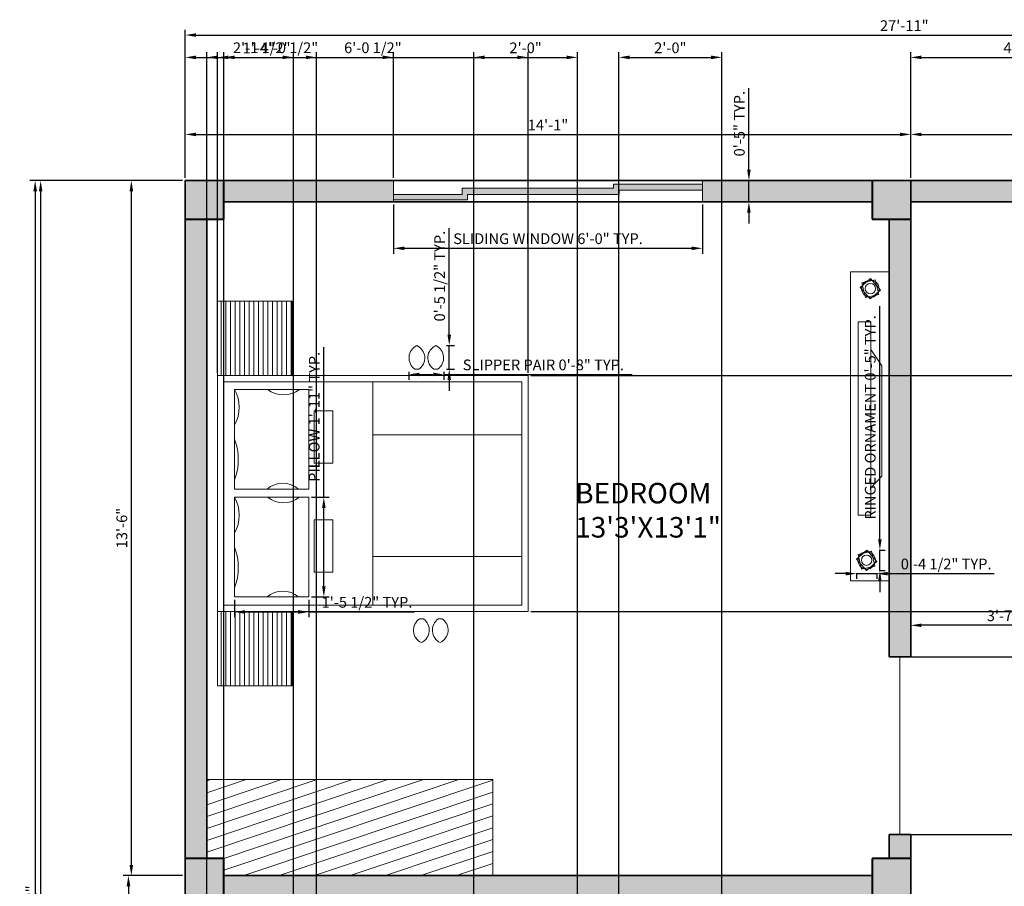
# Model space of a CAD drawing. Units: inches. Extents: x 918 to 1328, y 603 to 1174.
# Tile 3 of 4: x 918 to 1147, y 972 to 1174. Entities that reach past the tile are written whole.
import ezdxf

# ---------------------------------------------------------------- set-up
doc = ezdxf.new("R2010")
doc.units = ezdxf.units.IN
for name, color, linetype, lineweight in [('A-ANNO-DIMS', 1, 'Continuous', 18), ('A-COLS', 7, 'Continuous', 40), ('A-DOOR', 4, 'Continuous', 18), ('A-FLOR-CASE', 8, 'Continuous', 20), ('A-FURN', 8, 'Continuous', 18), ('A-FURN-PATT', 8, 'Continuous', 13), ('A-GLAZ', 4, 'Continuous', 18), ('A-GLAZ-PATT', 5, 'Continuous', 13), ('A-WALL', 7, 'Continuous', 35), ('A-WALL-PATT', 7, 'Continuous', 13)]:
    doc.layers.add(name, color=color, linetype=linetype, lineweight=lineweight)
for name, color, linetype, lineweight, true_color in [('A-AREA-IDEN', 251, 'Continuous', 20, 0x636466), ('A-COLS-PATT', 251, 'Continuous', 13, 0x636466), ('A-EQPM', 252, 'Continuous', 18, 0x939598), ('A-FLOR-CASE-PATT', 251, 'Continuous', 13, 0x636466)]:
    doc.layers.add(name, color=color, linetype=linetype, lineweight=lineweight, true_color=true_color)
doc.styles.get("Standard").update_dxf_attribs({"font": 'arial.ttf'})
doc.dimstyles.new('ISO-25', dxfattribs={"dimtxt": 2.5, "dimasz": 2.5, "dimexe": 1.25, "dimexo": 0.625, "dimtad": 1, "dimdec": 0, "dimlunit": 3, "dimtxsty": 'Standard', "dimcen": 2.5, "dimadec": 0, "dimazin": 0, "dimtfac": 1, "dimtdec": 0, "dimtmove": 0, "dimatfit": 3, "dimfxl": 1, "dimarcsym": 0})

# ---------------------------------------------------------------- blocks, each defined once
blk = doc.blocks.new('*D1')
at = {"layer": 'A-ANNO-DIMS', "color": 0, "lineweight": -2, "transparency": 16777216}
for p, q in [((956.48, 1136.87), (956.48, 1171.39)), ((958.98, 1170.14), (1288.98, 1170.14)), ((1291.48, 1136.87), (1291.48, 1171.39))]:
    blk.add_line(p, q, dxfattribs=at)
at = {"layer": 'A-ANNO-DIMS', "color": 0, "transparency": 16777216}
for points in [[(958.98, 1170.56), (958.98, 1169.73), (956.48, 1170.14)], [(1288.98, 1170.56), (1288.98, 1169.73), (1291.48, 1170.14)]]:
    blk.add_solid(points, dxfattribs=at)
at = {"layer": 'Defpoints', "color": 0, "transparency": 16777216}
for p in [(1291.48, 1170.14), (956.48, 1136.24), (1291.48, 1136.24)]:
    blk.add_point(p, dxfattribs=at)
at = {"layer": 'A-ANNO-DIMS', "color": 0, "transparency": 16777216, "insert": (1123.98, 1172.02), "char_height": 2.5, "attachment_point": 5}
blk.add_mtext('27\'-11"', dxfattribs=at)
blk = doc.blocks.new('*D2')
at = {"layer": 'A-ANNO-DIMS', "color": 0, "lineweight": -2, "transparency": 16777216}
for p, q in [((955.86, 1136.24), (921.53, 1136.24)), ((922.78, 1133.74), (922.78, 800.74)), ((955.86, 798.24), (921.53, 798.24))]:
    blk.add_line(p, q, dxfattribs=at)
at = {"layer": 'A-ANNO-DIMS', "color": 0, "transparency": 16777216}
for points in [[(922.37, 1133.74), (923.2, 1133.74), (922.78, 1136.24)], [(922.37, 800.74), (923.2, 800.74), (922.78, 798.24)]]:
    blk.add_solid(points, dxfattribs=at)
at = {"layer": 'Defpoints', "color": 0, "transparency": 16777216}
for p in [(956.48, 1136.24), (922.78, 798.24), (956.48, 798.24)]:
    blk.add_point(p, dxfattribs=at)
at = {"layer": 'A-ANNO-DIMS', "color": 0, "transparency": 16777216, "insert": (920.88, 967.24), "char_height": 2.5, "attachment_point": 5, "rotation": 90}
blk.add_mtext('28\'-2"', dxfattribs=at)
blk = doc.blocks.new('*D5')
at = {"layer": 'A-ANNO-DIMS', "color": 0, "lineweight": -2, "transparency": 16777216}
for p, q in [((1125.48, 1136.87), (1125.48, 1148.24)), ((1127.98, 1146.99), (1288.98, 1146.99)), ((1291.48, 1136.87), (1291.48, 1148.24))]:
    blk.add_line(p, q, dxfattribs=at)
at = {"layer": 'A-ANNO-DIMS', "color": 0, "transparency": 16777216}
for points in [[(1127.98, 1147.4), (1127.98, 1146.57), (1125.48, 1146.99)], [(1288.98, 1147.4), (1288.98, 1146.57), (1291.48, 1146.99)]]:
    blk.add_solid(points, dxfattribs=at)
at = {"layer": 'Defpoints', "color": 0, "transparency": 16777216}
for p in [(1291.48, 1146.99), (1125.48, 1136.24), (1291.48, 1136.24)]:
    blk.add_point(p, dxfattribs=at)
at = {"layer": 'A-ANNO-DIMS', "color": 0, "transparency": 16777216, "insert": (1208.48, 1148.89), "char_height": 2.5, "attachment_point": 5}
blk.add_mtext('13\'-10"', dxfattribs=at)
blk = doc.blocks.new('*D6')
at = {"layer": 'A-ANNO-DIMS', "color": 0, "lineweight": -2, "transparency": 16777216}
for p, q in [((956.48, 1136.87), (956.48, 1148.24)), ((958.98, 1146.99), (1122.98, 1146.99)), ((1125.48, 1136.87), (1125.48, 1148.24))]:
    blk.add_line(p, q, dxfattribs=at)
at = {"layer": 'A-ANNO-DIMS', "color": 0, "transparency": 16777216}
for points in [[(958.98, 1147.4), (958.98, 1146.57), (956.48, 1146.99)], [(1122.98, 1147.4), (1122.98, 1146.57), (1125.48, 1146.99)]]:
    blk.add_solid(points, dxfattribs=at)
at = {"layer": 'Defpoints', "color": 0, "transparency": 16777216}
for p in [(1125.48, 1146.99), (956.48, 1136.24), (1125.48, 1136.24)]:
    blk.add_point(p, dxfattribs=at)
at = {"layer": 'A-ANNO-DIMS', "color": 0, "transparency": 16777216, "insert": (1040.98, 1148.87), "char_height": 2.5, "attachment_point": 5}
blk.add_mtext('14\'-1"', dxfattribs=at)
blk = doc.blocks.new('*D7')
at = {"layer": 'A-ANNO-DIMS', "color": 0, "lineweight": -2, "transparency": 16777216}
for p, q in [((955.86, 1136.24), (942.66, 1136.24)), ((943.91, 976.74), (943.91, 1133.74)), ((955.86, 974.24), (942.66, 974.24))]:
    blk.add_line(p, q, dxfattribs=at)
at = {"layer": 'A-ANNO-DIMS', "color": 0, "transparency": 16777216}
for points in [[(943.49, 1133.74), (944.33, 1133.74), (943.91, 1136.24)], [(943.49, 976.74), (944.33, 976.74), (943.91, 974.24)]]:
    blk.add_solid(points, dxfattribs=at)
at = {"layer": 'Defpoints', "color": 0, "transparency": 16777216}
for p in [(943.91, 1136.24), (956.48, 1136.24), (956.48, 974.24)]:
    blk.add_point(p, dxfattribs=at)
at = {"layer": 'A-ANNO-DIMS', "color": 0, "transparency": 16777216, "insert": (942.01, 1055.24), "char_height": 2.5, "attachment_point": 5, "rotation": 90}
blk.add_mtext('13\'-6"', dxfattribs=at)
blk = doc.blocks.new('*D8')
at = {"layer": 'A-ANNO-DIMS', "color": 0, "lineweight": -2, "transparency": 16777216}
for p, q in [((955.86, 974.24), (941.99, 974.24)), ((943.24, 971.74), (943.24, 800.74)), ((955.86, 798.24), (941.99, 798.24))]:
    blk.add_line(p, q, dxfattribs=at)
at = {"layer": 'A-ANNO-DIMS', "color": 0, "transparency": 16777216}
for points in [[(942.82, 971.74), (943.66, 971.74), (943.24, 974.24)], [(942.82, 800.74), (943.66, 800.74), (943.24, 798.24)]]:
    blk.add_solid(points, dxfattribs=at)
at = {"layer": 'Defpoints', "color": 0, "transparency": 16777216}
for p in [(956.48, 974.24), (943.24, 798.24), (956.48, 798.24)]:
    blk.add_point(p, dxfattribs=at)
at = {"layer": 'A-ANNO-DIMS', "color": 0, "transparency": 16777216, "insert": (941.34, 886.24), "char_height": 2.5, "attachment_point": 5, "rotation": 90}
blk.add_mtext('14\'-8"', dxfattribs=at)
blk = doc.blocks.new('*D16')
at = {"layer": 'A-ANNO-DIMS', "color": 0, "lineweight": -2, "transparency": 16777216}
for p, q in [((1125.48, 1033.2), (1125.48, 1033.82)), ((1165.98, 1032.57), (1127.98, 1032.57)), ((1168.48, 1033.2), (1168.48, 1033.82))]:
    blk.add_line(p, q, dxfattribs=at)
at = {"layer": 'A-ANNO-DIMS', "color": 0, "transparency": 16777216}
for points in [[(1127.98, 1032.99), (1127.98, 1032.16), (1125.48, 1032.57)], [(1165.98, 1032.99), (1165.98, 1032.16), (1168.48, 1032.57)]]:
    blk.add_solid(points, dxfattribs=at)
at = {"layer": 'Defpoints', "color": 0, "transparency": 16777216}
for p in [(1125.48, 1032.57), (1125.48, 1032.57), (1168.48, 1032.57)]:
    blk.add_point(p, dxfattribs=at)
at = {"layer": 'A-ANNO-DIMS', "color": 0, "transparency": 16777216, "insert": (1146.98, 1034.48), "char_height": 2.5, "attachment_point": 5}
blk.add_mtext('3\'-7"', dxfattribs=at)
blk = doc.blocks.new('WIN-SLIDING-72')
for p, q in [((0, 5), (0, 0)), ((72, 5), (0, 5)), ((72, 0), (72, 5)), ((16, 3.25), (51.22, 3.25)), ((16, 3.25), (16, 1.76)), ((51.22, 4.12), (72, 4.12)), ((51.22, 3.25), (51.22, 4.12)), ((52.58, 2.76), (72, 2.76)), ((52.58, 1.76), (52.58, 2.76)), ((0, 1.76), (16, 1.76)), ((0, 0.47), (17.22, 0.47)), ((0, 0), (72, 0)), ((17.22, 1.76), (51.22, 1.76)), ((17.22, 1.76), (17.22, 0.47)), ((51.22, 1.76), (52.58, 1.76))]:
    blk.add_line(p, q)
blk = doc.blocks.new('PILLOW-BED')
blk.add_lwpolyline([(0, 0), (17.35, 0), (17.35, 23.25), (0, 23.25)], close=True)
for centre, radius, start, end in [((-7.16, 19.07), 8.29, 329.7831, 30.2169), ((11.43, 28.01), 6.06, 231.8235, 308.1765), ((-11.88, 6.88), 12.79, 338.2152, 21.7848), ((11.27, -4.17), 5.55, 48.6314, 131.3686)]:
    blk.add_arc(centre, radius, start, end)
blk = doc.blocks.new('SLIPPERS-PAIR')
for p, q in [((1.4, 0), (2.26, 0)), ((5.79, 0), (6.66, 0))]:
    blk.add_line(p, q)
for centre, start, end in [((3.2, 2.65), 115.3264, 235.7805), ((0.46, 2.65), 304.2195, 64.6736), ((7.59, 2.65), 115.3264, 235.7805), ((4.86, 2.65), 304.2195, 64.6736)]:
    blk.add_arc(centre, 3.2, start, end)
blk = doc.blocks.new('CONSOLE-ORNAMENT-RINGED')
for p, q in [((2.4, 4.76), (0, 2.68)), ((4.73, 2.08), (2.4, 4.76)), ((0, 2.68), (2.33, 0)), ((3.48, 4.49), (0.38, 3.76)), ((0.38, 3.76), (1.19, 0.31)), ((4.29, 1.03), (3.48, 4.49)), ((1.19, 0.31), (4.29, 1.03)), ((2.33, 0), (4.73, 2.08))]:
    blk.add_line(p, q)
for centre, radius in [((2.36, 2.38), 2.02), ((2.35, 2.42), 1.21)]:
    blk.add_circle(centre, radius)
blk = doc.blocks.new('*D30')
at = {"layer": 'A-ANNO-DIMS', "color": 0, "lineweight": -2, "transparency": 16777216}
for p, q in [((1004.98, 1130.62), (1004.98, 1119.19)), ((1076.98, 1130.62), (1076.98, 1119.19)), ((1007.48, 1120.44), (1074.48, 1120.44))]:
    blk.add_line(p, q, dxfattribs=at)
at = {"layer": 'A-ANNO-DIMS', "color": 0, "transparency": 16777216}
for points in [[(1007.48, 1120.86), (1007.48, 1120.03), (1004.98, 1120.44)], [(1074.48, 1120.86), (1074.48, 1120.03), (1076.98, 1120.44)]]:
    blk.add_solid(points, dxfattribs=at)
at = {"layer": 'Defpoints', "color": 0, "transparency": 16777216}
for p in [(1004.98, 1131.24), (1076.98, 1131.24), (1076.98, 1120.44)]:
    blk.add_point(p, dxfattribs=at)
at = {"layer": 'A-ANNO-DIMS', "color": 0, "transparency": 16777216, "insert": (1040.98, 1122.36), "char_height": 2.5, "attachment_point": 5}
blk.add_mtext('SLIDING WINDOW 6\'-0" TYP.', dxfattribs=at)
blk = doc.blocks.new('*D31')
at = {"layer": 'A-ANNO-DIMS', "color": 0, "lineweight": -2, "transparency": 16777216}
for p, q in [((1087.78, 1138.74), (1087.78, 1157.73)), ((1077.61, 1136.24), (1089.03, 1136.24)), ((1087.78, 1131.24), (1087.78, 1136.24)), ((1077.61, 1131.24), (1089.03, 1131.24)), ((1087.78, 1128.74), (1087.78, 1126.24))]:
    blk.add_line(p, q, dxfattribs=at)
at = {"layer": 'A-ANNO-DIMS', "color": 0, "transparency": 16777216}
for points in [[(1087.37, 1138.74), (1088.2, 1138.74), (1087.78, 1136.24)], [(1087.37, 1128.74), (1088.2, 1128.74), (1087.78, 1131.24)]]:
    blk.add_solid(points, dxfattribs=at)
at = {"layer": 'Defpoints', "color": 0, "transparency": 16777216}
for p in [(1076.98, 1136.24), (1087.78, 1136.24), (1076.98, 1131.24)]:
    blk.add_point(p, dxfattribs=at)
at = {"layer": 'A-ANNO-DIMS', "color": 0, "transparency": 16777216, "insert": (1085.88, 1149.49), "char_height": 2.5, "attachment_point": 5, "rotation": 90}
blk.add_mtext('0\'-5" TYP.', dxfattribs=at)
blk = doc.blocks.new('*D36')
at = {"layer": 'A-ANNO-DIMS', "color": 0, "lineweight": -2, "transparency": 16777216}
for p, q in [((988.75, 1062.42), (988.75, 1097.4)), ((985.89, 1062.42), (990, 1062.42)), ((988.75, 1041.68), (988.75, 1059.92)), ((985.89, 1039.18), (990, 1039.18))]:
    blk.add_line(p, q, dxfattribs=at)
at = {"layer": 'A-ANNO-DIMS', "color": 0, "transparency": 16777216}
for points in [[(988.34, 1059.92), (989.17, 1059.92), (988.75, 1062.42)], [(988.34, 1041.68), (989.17, 1041.68), (988.75, 1039.18)]]:
    blk.add_solid(points, dxfattribs=at)
at = {"layer": 'Defpoints', "color": 0, "transparency": 16777216}
for p in [(985.27, 1062.42), (988.75, 1062.42), (985.27, 1039.18)]:
    blk.add_point(p, dxfattribs=at)
at = {"layer": 'A-ANNO-DIMS', "color": 0, "transparency": 16777216, "insert": (986.84, 1081.16), "char_height": 2.5, "attachment_point": 5, "rotation": 90}
blk.add_mtext('PILLOW 1\'-11" TYP.', dxfattribs=at)
blk = doc.blocks.new('*D37')
at = {"layer": 'A-ANNO-DIMS', "color": 0, "lineweight": -2, "transparency": 16777216}
for p, q in [((967.92, 1038.55), (967.92, 1034.44)), ((985.27, 1038.55), (985.27, 1034.44)), ((970.42, 1035.69), (982.77, 1035.69)), ((985.27, 1035.69), (1009.85, 1035.69))]:
    blk.add_line(p, q, dxfattribs=at)
at = {"layer": 'A-ANNO-DIMS', "color": 0, "transparency": 16777216}
for points in [[(970.42, 1036.11), (970.42, 1035.27), (967.92, 1035.69)], [(982.77, 1036.11), (982.77, 1035.27), (985.27, 1035.69)]]:
    blk.add_solid(points, dxfattribs=at)
at = {"layer": 'Defpoints', "color": 0, "transparency": 16777216}
for p in [(967.92, 1039.18), (985.27, 1039.18), (985.27, 1035.69)]:
    blk.add_point(p, dxfattribs=at)
at = {"layer": 'A-ANNO-DIMS', "color": 0, "transparency": 16777216, "insert": (998.81, 1037.61), "char_height": 2.5, "attachment_point": 5}
blk.add_mtext('1\'-5 1/2" TYP.', dxfattribs=at)
blk = doc.blocks.new('*D38')
at = {"layer": 'A-ANNO-DIMS', "color": 0, "lineweight": -2, "transparency": 16777216}
for p, q in [((1008.52, 1091.64), (1008.52, 1089.78)), ((1011.02, 1091.03), (1014.24, 1091.03)), ((1016.74, 1091.64), (1016.74, 1089.78)), ((1016.74, 1091.03), (1060.56, 1091.03))]:
    blk.add_line(p, q, dxfattribs=at)
at = {"layer": 'A-ANNO-DIMS', "color": 0, "transparency": 16777216}
for points in [[(1011.02, 1091.45), (1011.02, 1090.61), (1008.52, 1091.03)], [(1014.24, 1091.45), (1014.24, 1090.61), (1016.74, 1091.03)]]:
    blk.add_solid(points, dxfattribs=at)
at = {"layer": 'Defpoints', "color": 0, "transparency": 16777216}
for p in [(1008.52, 1092.26), (1016.74, 1092.26), (1016.74, 1091.03)]:
    blk.add_point(p, dxfattribs=at)
at = {"layer": 'A-ANNO-DIMS', "color": 0, "transparency": 16777216, "insert": (1039.9, 1092.95), "char_height": 2.5, "attachment_point": 5}
blk.add_mtext('SLIPPER PAIR 0\'-8" TYP.', dxfattribs=at)
blk = doc.blocks.new('*D39')
at = {"layer": 'A-ANNO-DIMS', "color": 0, "lineweight": -2, "transparency": 16777216}
for p, q in [((1017.97, 1100.3), (1017.97, 1125.12)), ((1017.36, 1097.8), (1019.22, 1097.8)), ((1017.97, 1092.26), (1017.97, 1097.8)), ((1017.36, 1092.26), (1019.22, 1092.26)), ((1017.97, 1089.76), (1017.97, 1087.26))]:
    blk.add_line(p, q, dxfattribs=at)
at = {"layer": 'A-ANNO-DIMS', "color": 0, "transparency": 16777216}
for points in [[(1017.55, 1100.3), (1018.39, 1100.3), (1017.97, 1097.8)], [(1017.55, 1089.76), (1018.39, 1089.76), (1017.97, 1092.26)]]:
    blk.add_solid(points, dxfattribs=at)
at = {"layer": 'Defpoints', "color": 0, "transparency": 16777216}
for p in [(1016.74, 1097.8), (1017.97, 1097.8), (1016.74, 1092.26)]:
    blk.add_point(p, dxfattribs=at)
at = {"layer": 'A-ANNO-DIMS', "color": 0, "transparency": 16777216, "insert": (1016.05, 1113.96), "char_height": 2.5, "attachment_point": 5, "rotation": 90}
blk.add_mtext('0\'-5 1/2" TYP.', dxfattribs=at)
blk = doc.blocks.new('*D40')
at = {"layer": 'A-ANNO-DIMS', "color": 0, "lineweight": -2, "transparency": 16777216}
for p, q in [((1118.3, 1052.6), (1118.3, 1106.97)), ((1118.21, 1050.1), (1119.55, 1050.1)), ((1118.3, 1045.33), (1118.3, 1050.1)), ((1118.21, 1045.33), (1119.55, 1045.33)), ((1118.3, 1042.83), (1118.3, 1040.33))]:
    blk.add_line(p, q, dxfattribs=at)
at = {"layer": 'A-ANNO-DIMS', "color": 0, "transparency": 16777216}
for points in [[(1117.88, 1052.6), (1118.71, 1052.6), (1118.3, 1050.1)], [(1117.88, 1042.83), (1118.71, 1042.83), (1118.3, 1045.33)]]:
    blk.add_solid(points, dxfattribs=at)
at = {"layer": 'Defpoints', "color": 0, "transparency": 16777216}
for p in [(1117.58, 1050.1), (1118.3, 1050.1), (1117.58, 1045.33)]:
    blk.add_point(p, dxfattribs=at)
at = {"layer": 'A-ANNO-DIMS', "color": 0, "transparency": 16777216, "insert": (1116.38, 1081.03), "char_height": 2.5, "attachment_point": 5, "rotation": 90}
blk.add_mtext('RINGED ORNAMENT 0\'-5" TYP.', dxfattribs=at)
blk = doc.blocks.new('*D41')
at = {"layer": 'A-ANNO-DIMS', "color": 0, "lineweight": -2, "transparency": 16777216}
for p, q in [((1110.36, 1044.62), (1107.86, 1044.62)), ((1112.86, 1044.71), (1112.86, 1043.37)), ((1112.86, 1044.62), (1117.58, 1044.62)), ((1117.58, 1044.71), (1117.58, 1043.37)), ((1120.08, 1044.62), (1144.9, 1044.62))]:
    blk.add_line(p, q, dxfattribs=at)
at = {"layer": 'A-ANNO-DIMS', "color": 0, "transparency": 16777216}
for points in [[(1110.36, 1045.04), (1110.36, 1044.2), (1112.86, 1044.62)], [(1120.08, 1045.04), (1120.08, 1044.2), (1117.58, 1044.62)]]:
    blk.add_solid(points, dxfattribs=at)
at = {"layer": 'Defpoints', "color": 0, "transparency": 16777216}
for p in [(1112.86, 1045.33), (1117.58, 1045.33), (1117.58, 1044.62)]:
    blk.add_point(p, dxfattribs=at)
at = {"layer": 'A-ANNO-DIMS', "color": 0, "transparency": 16777216, "insert": (1133.74, 1046.54), "char_height": 2.5, "attachment_point": 5}
blk.add_mtext('0\'-4 1/2" TYP.', dxfattribs=at)
blk = doc.blocks.new('*D44')
at = {"layer": 'A-ANNO-DIMS', "color": 0, "lineweight": -2, "transparency": 16777216}
for p, q in [((955.86, 1136.24), (920.25, 1136.24)), ((921.5, 1133.74), (921.5, 731.74)), ((1064.86, 729.24), (920.25, 729.24))]:
    blk.add_line(p, q, dxfattribs=at)
at = {"layer": 'A-ANNO-DIMS', "color": 0, "transparency": 16777216}
for points in [[(921.09, 1133.74), (921.92, 1133.74), (921.5, 1136.24)], [(921.09, 731.74), (921.92, 731.74), (921.5, 729.24)]]:
    blk.add_solid(points, dxfattribs=at)
at = {"layer": 'Defpoints', "color": 0, "transparency": 16777216}
for p in [(956.48, 1136.24), (921.5, 729.24), (1065.48, 729.24)]:
    blk.add_point(p, dxfattribs=at)
at = {"layer": 'A-ANNO-DIMS', "color": 0, "transparency": 16777216, "insert": (919.6, 932.74), "char_height": 2.5, "attachment_point": 5, "rotation": 90}
blk.add_mtext('33\'-11"', dxfattribs=at)
blk = doc.blocks.new('*D45')
at = {"layer": 'A-ANNO-DIMS', "color": 0, "lineweight": -2, "transparency": 16777216}
for p, q in [((956.48, 1136.87), (956.48, 1166.19)), ((1004.98, 1136.87), (1004.98, 1166.19)), ((958.98, 1164.94), (1002.48, 1164.94))]:
    blk.add_line(p, q, dxfattribs=at)
at = {"layer": 'A-ANNO-DIMS', "color": 0, "transparency": 16777216}
for points in [[(958.98, 1165.36), (958.98, 1164.53), (956.48, 1164.94)], [(1002.48, 1165.36), (1002.48, 1164.53), (1004.98, 1164.94)]]:
    blk.add_solid(points, dxfattribs=at)
at = {"layer": 'Defpoints', "color": 0, "transparency": 16777216}
for p in [(1004.98, 1164.94), (956.48, 1136.24), (1004.98, 1136.24)]:
    blk.add_point(p, dxfattribs=at)
at = {"layer": 'A-ANNO-DIMS', "color": 0, "transparency": 16777216, "insert": (980.73, 1166.86), "char_height": 2.5, "attachment_point": 5}
blk.add_mtext('4\'-0 1/2"', dxfattribs=at)
blk = doc.blocks.new('*D46')
at = {"layer": 'A-ANNO-DIMS', "color": 0, "lineweight": -2, "transparency": 16777216}
for p, q in [((1125.48, 1136.87), (1125.48, 1166.19)), ((1176.26, 1136.87), (1176.26, 1166.19)), ((1127.98, 1164.94), (1173.76, 1164.94))]:
    blk.add_line(p, q, dxfattribs=at)
at = {"layer": 'A-ANNO-DIMS', "color": 0, "transparency": 16777216}
for points in [[(1127.98, 1165.36), (1127.98, 1164.53), (1125.48, 1164.94)], [(1173.76, 1165.36), (1173.76, 1164.53), (1176.26, 1164.94)]]:
    blk.add_solid(points, dxfattribs=at)
at = {"layer": 'Defpoints', "color": 0, "transparency": 16777216}
for p in [(1176.26, 1164.94), (1125.48, 1136.24), (1176.26, 1136.24)]:
    blk.add_point(p, dxfattribs=at)
at = {"layer": 'A-ANNO-DIMS', "color": 0, "transparency": 16777216, "insert": (1150.87, 1166.84), "char_height": 2.5, "attachment_point": 5}
blk.add_mtext('4\'-3"', dxfattribs=at)
blk = doc.blocks.new('*D47')
at = {"layer": 'A-ANNO-DIMS', "color": 0, "lineweight": -2, "transparency": 16777216}
for p, q in [((965.48, 803.87), (965.48, 1166.19)), ((981.69, 803.87), (981.69, 1166.19)), ((967.98, 1164.94), (979.19, 1164.94))]:
    blk.add_line(p, q, dxfattribs=at)
at = {"layer": 'A-ANNO-DIMS', "color": 0, "transparency": 16777216}
for points in [[(967.98, 1165.36), (967.98, 1164.53), (965.48, 1164.94)], [(979.19, 1165.36), (979.19, 1164.53), (981.69, 1164.94)]]:
    blk.add_solid(points, dxfattribs=at)
at = {"layer": 'Defpoints', "color": 0, "transparency": 16777216}
for p in [(981.69, 1164.94), (965.48, 803.24), (981.69, 803.24)]:
    blk.add_point(p, dxfattribs=at)
at = {"layer": 'A-ANNO-DIMS', "color": 0, "transparency": 16777216, "insert": (973.59, 1166.82), "char_height": 2.5, "attachment_point": 5}
blk.add_mtext('1\'-4"', dxfattribs=at)
blk = doc.blocks.new('*D48')
at = {"layer": 'A-ANNO-DIMS', "color": 0, "lineweight": -2, "transparency": 16777216}
for p, q in [((1023.69, 803.87), (1023.69, 1166.19)), ((1047.83, 803.87), (1047.83, 1166.19)), ((1026.19, 1164.94), (1045.33, 1164.94))]:
    blk.add_line(p, q, dxfattribs=at)
at = {"layer": 'A-ANNO-DIMS', "color": 0, "transparency": 16777216}
for points in [[(1026.19, 1165.36), (1026.19, 1164.53), (1023.69, 1164.94)], [(1045.33, 1165.36), (1045.33, 1164.53), (1047.83, 1164.94)]]:
    blk.add_solid(points, dxfattribs=at)
at = {"layer": 'Defpoints', "color": 0, "transparency": 16777216}
for p in [(1047.83, 1164.94), (1023.69, 803.24), (1047.83, 803.24)]:
    blk.add_point(p, dxfattribs=at)
at = {"layer": 'A-ANNO-DIMS', "color": 0, "transparency": 16777216, "insert": (1035.76, 1166.84), "char_height": 2.5, "attachment_point": 5}
blk.add_mtext('2\'-0"', dxfattribs=at)
blk = doc.blocks.new('*D50')
at = {"layer": 'A-ANNO-DIMS', "color": 0, "lineweight": -2, "transparency": 16777216}
for p, q in [((1121.11, 1025.24), (1321.43, 1025.24)), ((1320.18, 1022.74), (1320.18, 986.29)), ((1121.11, 983.79), (1321.43, 983.79))]:
    blk.add_line(p, q, dxfattribs=at)
at = {"layer": 'A-ANNO-DIMS', "color": 0, "transparency": 16777216}
for points in [[(1319.77, 1022.74), (1320.6, 1022.74), (1320.18, 1025.24)], [(1319.77, 986.29), (1320.6, 986.29), (1320.18, 983.79)]]:
    blk.add_solid(points, dxfattribs=at)
at = {"layer": 'Defpoints', "color": 0, "transparency": 16777216}
for p in [(1120.48, 1025.24), (1120.48, 983.79), (1320.18, 983.79)]:
    blk.add_point(p, dxfattribs=at)
at = {"layer": 'A-ANNO-DIMS', "color": 0, "transparency": 16777216, "insert": (1318.26, 1004.52), "char_height": 2.5, "attachment_point": 5, "rotation": 90}
blk.add_mtext('3\'-5 1/2"', dxfattribs=at)
blk = doc.blocks.new('*D52')
at = {"layer": 'A-ANNO-DIMS', "color": 0, "lineweight": -2, "transparency": 16777216}
for p, q in [((964.01, 1091.42), (964.01, 1166.19)), ((1036.36, 1091.42), (1036.36, 1166.19)), ((966.51, 1164.94), (1033.86, 1164.94))]:
    blk.add_line(p, q, dxfattribs=at)
at = {"layer": 'A-ANNO-DIMS', "color": 0, "transparency": 16777216}
for points in [[(966.51, 1165.36), (966.51, 1164.53), (964.01, 1164.94)], [(1033.86, 1165.36), (1033.86, 1164.53), (1036.36, 1164.94)]]:
    blk.add_solid(points, dxfattribs=at)
at = {"layer": 'Defpoints', "color": 0, "transparency": 16777216}
for p in [(1036.36, 1164.94), (964.01, 1090.79), (1036.36, 1090.79)]:
    blk.add_point(p, dxfattribs=at)
at = {"layer": 'A-ANNO-DIMS', "color": 0, "transparency": 16777216, "insert": (1000.18, 1166.86), "char_height": 2.5, "attachment_point": 5}
blk.add_mtext('6\'-0 1/2"', dxfattribs=at)
blk = doc.blocks.new('*D53')
at = {"layer": 'A-ANNO-DIMS', "color": 0, "lineweight": -2, "transparency": 16777216}
for p, q in [((1036.99, 1090.79), (1321.43, 1090.79)), ((1320.18, 1038.3), (1320.18, 1088.29)), ((1036.99, 1035.8), (1321.43, 1035.8))]:
    blk.add_line(p, q, dxfattribs=at)
at = {"layer": 'A-ANNO-DIMS', "color": 0, "transparency": 16777216}
for points in [[(1319.77, 1088.29), (1320.6, 1088.29), (1320.18, 1090.79)], [(1319.77, 1038.3), (1320.6, 1038.3), (1320.18, 1035.8)]]:
    blk.add_solid(points, dxfattribs=at)
at = {"layer": 'Defpoints', "color": 0, "transparency": 16777216}
for p in [(1036.36, 1090.79), (1320.18, 1090.79), (1036.36, 1035.8)]:
    blk.add_point(p, dxfattribs=at)
at = {"layer": 'A-ANNO-DIMS', "color": 0, "transparency": 16777216, "insert": (1318.31, 1063.3), "char_height": 2.5, "attachment_point": 5, "rotation": 90}
blk.add_mtext('4\'-7"', dxfattribs=at)
blk = doc.blocks.new('*D54')
at = {"layer": 'A-ANNO-DIMS', "color": 0, "lineweight": -2, "transparency": 16777216}
for p, q in [((961.48, 868.87), (961.48, 1166.19)), ((987.08, 868.87), (987.08, 1166.19)), ((963.98, 1164.94), (984.58, 1164.94))]:
    blk.add_line(p, q, dxfattribs=at)
at = {"layer": 'A-ANNO-DIMS', "color": 0, "transparency": 16777216}
for points in [[(963.98, 1165.36), (963.98, 1164.53), (961.48, 1164.94)], [(984.58, 1165.36), (984.58, 1164.53), (987.08, 1164.94)]]:
    blk.add_solid(points, dxfattribs=at)
at = {"layer": 'Defpoints', "color": 0, "transparency": 16777216}
for p in [(987.08, 1164.94), (961.48, 868.24), (987.08, 868.24)]:
    blk.add_point(p, dxfattribs=at)
at = {"layer": 'A-ANNO-DIMS', "color": 0, "transparency": 16777216, "insert": (974.28, 1166.86), "char_height": 2.5, "attachment_point": 5}
blk.add_mtext('2\'-1 1/2"', dxfattribs=at)
blk = doc.blocks.new('*D55')
at = {"layer": 'A-ANNO-DIMS', "color": 0, "lineweight": -2, "transparency": 16777216}
for p, q in [((1057.48, 856.87), (1057.48, 1166.19)), ((1081.48, 856.87), (1081.48, 1166.19)), ((1059.98, 1164.94), (1078.98, 1164.94))]:
    blk.add_line(p, q, dxfattribs=at)
at = {"layer": 'A-ANNO-DIMS', "color": 0, "transparency": 16777216}
for points in [[(1059.98, 1165.36), (1059.98, 1164.53), (1057.48, 1164.94)], [(1078.98, 1165.36), (1078.98, 1164.53), (1081.48, 1164.94)]]:
    blk.add_solid(points, dxfattribs=at)
at = {"layer": 'Defpoints', "color": 0, "transparency": 16777216}
for p in [(1081.48, 1164.94), (1057.48, 856.24), (1081.48, 856.24)]:
    blk.add_point(p, dxfattribs=at)
at = {"layer": 'A-ANNO-DIMS', "color": 0, "transparency": 16777216, "insert": (1069.48, 1166.84), "char_height": 2.5, "attachment_point": 5}
blk.add_mtext('2\'-0"', dxfattribs=at)

msp = doc.modelspace()

# ---------------------------------------------------------------- hatches: boundary and pattern name
at = {"layer": 'A-COLS-PATT'}
h = msp.add_hatch(color=256, dxfattribs=at)
h.dxf.hatch_style = 1
h.paths.add_polyline_path([(965.48, 1136.24), (956.48, 1136.24), (956.48, 1127.24), (965.48, 1127.24)])
h.paths.add_polyline_path([(1125.48, 1136.24), (1116.48, 1136.24), (1116.48, 1127.24), (1125.48, 1127.24)])
h.paths.add_polyline_path([(1291.48, 1136.24), (1282.48, 1136.24), (1282.48, 1127.24), (1291.48, 1127.24)])
h.paths.add_polyline_path([(1125.48, 978.24), (1116.48, 978.24), (1116.48, 969.24), (1125.48, 969.24)])
h.paths.add_polyline_path([(965.48, 978.24), (956.48, 978.24), (956.48, 969.24), (965.48, 969.24)])
h.paths.add_polyline_path([(965.48, 807.24), (956.48, 807.24), (956.48, 798.24), (965.48, 798.24)])
h.paths.add_polyline_path([(1125.48, 807.24), (1116.48, 807.24), (1116.48, 798.24), (1125.48, 798.24)])
h.paths.add_polyline_path([(1291.48, 807.24), (1282.48, 807.24), (1282.48, 798.24), (1291.48, 798.24)])
h.paths.add_polyline_path([(1291.48, 1030.24), (1282.48, 1030.24), (1282.48, 1021.24), (1291.48, 1021.24)])
h.paths.add_polyline_path([(1291.48, 978.24), (1282.48, 978.24), (1282.48, 969.24), (1291.48, 969.24)])
at = {"layer": 'A-FLOR-CASE-PATT'}
h = msp.add_hatch(dxfattribs=at)
h.set_pattern_fill('ANSI31', color=256, scale=0.827794, angle=-26.45, style=0)
h.paths.add_polyline_path([(961.48, 978.24), (965.48, 978.24), (965.48, 974.24), (1028.14, 974.24), (1028.14, 996.61), (961.48, 996.61)])
at = {"layer": 'A-FURN-PATT'}
h = msp.add_hatch(dxfattribs=at)
h.set_pattern_fill('ANSI31', color=256, scale=0.3418386, angle=45, style=0)
h.paths.add_polyline_path([(964.01, 1090.79), (981.37, 1090.79), (981.37, 1108.16), (964.01, 1108.16)])
h = msp.add_hatch(dxfattribs=at)
h.set_pattern_fill('ANSI31', color=256, scale=0.3418386, angle=45, style=0)
h.paths.add_polyline_path([(964.01, 1018.44), (981.37, 1018.44), (981.37, 1035.8), (964.01, 1035.8)])
at = {"layer": 'A-GLAZ-PATT'}
h = msp.add_hatch(color=256, dxfattribs=at)
h.dxf.hatch_style = 1
h.paths.add_polyline_path([(1057.57, 1134.01), (1076.98, 1134.01), (1076.98, 1135.36), (1056.2, 1135.36), (1056.2, 1134.49), (1020.98, 1134.49), (1020.98, 1133), (1004.98, 1133), (1004.98, 1131.71), (1022.21, 1131.71), (1022.21, 1133), (1056.21, 1133), (1057.57, 1133)])
h.paths.add_polyline_path([(1228.84, 1134.01), (1248.26, 1134.01), (1248.26, 1135.36), (1227.48, 1135.36), (1227.48, 1134.49), (1192.26, 1134.49), (1192.26, 1133), (1176.26, 1133), (1176.26, 1131.71), (1193.48, 1131.71), (1193.48, 1133), (1227.48, 1133), (1228.84, 1133)])
h.paths.add_polyline_path([(1244.5, 828.01), (1263.92, 828.01), (1263.92, 829.36), (1243.14, 829.36), (1243.14, 828.49), (1207.92, 828.49), (1207.92, 827), (1191.92, 827), (1191.92, 825.71), (1209.14, 825.71), (1209.14, 827), (1243.14, 827), (1244.5, 827)])
at = {"layer": 'A-WALL-PATT'}
h = msp.add_hatch(color=256, dxfattribs=at)
h.dxf.hatch_style = 1
h.paths.add_polyline_path([(961.48, 969.24), (956.48, 969.24), (956.48, 807.24), (961.48, 807.24), (961.48, 904.24), (1125.48, 904.24), (1125.48, 909.24), (1086.48, 909.24), (1086.48, 913.24), (1081.48, 913.24), (1081.48, 909.24), (961.48, 909.24)])
h.paths.add_polyline_path([(1116.48, 974.24), (965.48, 974.24), (965.48, 969.24), (1081.48, 969.24), (1081.48, 943.24), (1086.48, 943.24), (1086.48, 969.24), (1116.48, 969.24)])
h.paths.add_polyline_path([(1004.98, 1136.24), (965.48, 1136.24), (965.48, 1131.24), (1004.98, 1131.24)])
h.paths.add_polyline_path([(1116.48, 1136.24), (1076.98, 1136.24), (1076.98, 1131.24), (1116.48, 1131.24)])
h.paths.add_polyline_path([(1176.26, 1136.24), (1125.48, 1136.24), (1125.48, 1131.24), (1176.26, 1131.24)])
h.paths.add_polyline_path([(1282.48, 1136.24), (1248.26, 1136.24), (1248.26, 1131.24), (1282.48, 1131.24)])
h.paths.add_polyline_path([(1125.48, 1127.24), (1120.48, 1127.24), (1120.48, 1025.24), (1125.48, 1025.24)])
h.paths.add_polyline_path([(1291.48, 1035.24), (1168.48, 1035.24), (1168.48, 1030.24), (1291.48, 1030.24)])
h.paths.add_polyline_path([(1125.48, 825.24), (1129.48, 825.24), (1129.48, 830.24), (1125.48, 830.24), (1125.48, 856.24), (1120.48, 856.24), (1120.48, 807.24), (1125.48, 807.24)])
h.paths.add_polyline_path([(1191.92, 830.24), (1177.48, 830.24), (1177.48, 825.24), (1191.92, 825.24)])
h.paths.add_polyline_path([(1291.48, 969.24), (1286.48, 969.24), (1286.48, 830.24), (1263.92, 830.24), (1263.92, 825.24), (1286.48, 825.24), (1286.48, 807.24), (1291.48, 807.24)])
h.paths.add_polyline_path([(1291.48, 1021.24), (1286.48, 1021.24), (1286.48, 978.24), (1291.48, 978.24)])
h.paths.add_polyline_path([(1291.48, 1127.24), (1286.48, 1127.24), (1286.48, 1035.24), (1291.48, 1035.24)])
h = msp.add_hatch(color=256, dxfattribs=at)
h.dxf.hatch_style = 1
h.paths.add_polyline_path([(961.48, 1127.24), (956.48, 1127.24), (956.48, 978.24), (961.48, 978.24), (961.48, 996.61)])
h = msp.add_hatch(color=256, dxfattribs=at)
h.dxf.hatch_style = 1
h.paths.add_polyline_path([(1125.48, 983.79), (1120.48, 983.79), (1120.48, 978.24), (1125.48, 978.24)])

# ---------------------------------------------------------------- linework, layer by layer
at = {"layer": 'A-COLS'}
for p, q in [((965.48, 1127.24), (965.48, 1136.24)), ((1116.48, 1136.24), (1116.48, 1127.24)), ((956.48, 1127.24), (965.48, 1127.24)), ((1116.48, 1127.24), (1125.48, 1127.24)), ((965.48, 978.24), (956.48, 978.24)), ((965.48, 969.24), (965.48, 978.24)), ((1125.48, 978.24), (1116.48, 978.24)), ((1116.48, 978.24), (1116.48, 969.24))]:
    msp.add_line(p, q, dxfattribs=at)
at = {"layer": 'A-DOOR'}
msp.add_line((1122.98, 983.79), (1122.98, 1025.24), dxfattribs=at)
at = {"layer": 'A-EQPM'}
for p, q in [((1116.16, 1103.3), (1113.21, 1103.3)), ((1113.21, 1103.3), (1113.21, 1058.22)), ((1116.16, 1058.22), (1116.16, 1103.3)), ((1116.16, 1096.89), (1118.76, 1093.02)), ((1118.76, 1093.02), (1118.76, 1067.31)), ((1118.76, 1067.31), (1116.16, 1064.61)), ((1113.21, 1058.22), (1116.16, 1058.22))]:
    msp.add_line(p, q, dxfattribs=at)
at = {"layer": 'A-FLOR-CASE'}
for p, q in [((1120.48, 1114.95), (1111.48, 1114.95)), ((1111.48, 1114.95), (1111.48, 1042.95)), ((1120.48, 1042.95), (1120.48, 1114.95)), ((1111.48, 1042.95), (1120.48, 1042.95)), ((961.48, 996.61), (961.48, 978.24)), ((1028.14, 996.61), (961.48, 996.61)), ((1028.14, 974.24), (1028.14, 996.61)), ((965.48, 974.24), (1028.14, 974.24))]:
    msp.add_line(p, q, dxfattribs=at)
at = {"layer": 'A-FURN'}
for p, q in [((1000.18, 1089.35), (1000.18, 1037.25)), ((976.99, 1035.8), (964.01, 1035.8)), ((964.01, 1035.8), (964.01, 1018.44)), ((981.37, 1035.8), (981.37, 1018.44)), ((964.01, 1018.44), (981.37, 1018.44))]:
    msp.add_line(p, q, dxfattribs=at)
for points in [[(964.01, 1090.79), (981.37, 1090.79), (981.37, 1108.16), (964.01, 1108.16)], [(964.01, 1090.79), (964.01, 1035.8), (1036.36, 1035.8), (1036.36, 1090.79)], [(965.45, 1089.35), (965.45, 1037.25), (1034.92, 1037.25), (1034.92, 1089.35)], [(986.47, 1082.56), (990.88, 1082.56), (990.88, 1070.33), (986.47, 1070.33)], [(1034.92, 1076.95), (1000.18, 1076.95), (1000.18, 1076.95), (1034.92, 1076.95)], [(986.47, 1057.19), (990.88, 1057.19), (990.88, 1044.97), (986.47, 1044.97)], [(1034.92, 1048.6), (1000.18, 1048.6), (1000.18, 1048.6), (1034.92, 1048.6)]]:
    msp.add_lwpolyline(points, close=True, dxfattribs=at)
at = {"layer": 'A-WALL'}
for p, q in [((1291.48, 1136.24), (956.48, 1136.24)), ((956.48, 1136.24), (956.48, 798.24)), ((1125.48, 1136.24), (1125.48, 1025.24)), ((1116.48, 1131.24), (965.48, 1131.24)), ((1282.48, 1131.24), (1125.48, 1131.24)), ((961.48, 1127.24), (961.48, 978.24)), ((1120.48, 1127.24), (1120.48, 1025.24)), ((1125.48, 1025.24), (1120.48, 1025.24)), ((1120.48, 983.79), (1125.48, 983.79)), ((1120.48, 983.79), (1120.48, 978.24)), ((1125.48, 983.79), (1125.48, 969.24)), ((1116.48, 974.24), (965.48, 974.24))]:
    msp.add_line(p, q, dxfattribs=at)

# ---------------------------------------------------------------- block references
at = {"layer": 'A-FURN'}
for name, p in [('CONSOLE-ORNAMENT-RINGED', (1113.73, 1108.64)), ('SLIPPERS-PAIR', (1008.6, 1092.26)), ('PILLOW-BED', (967.92, 1064.32)), ('PILLOW-BED', (967.92, 1039.18)), ('CONSOLE-ORNAMENT-RINGED', (1112.86, 1045.33))]:
    msp.add_blockref(name, p, dxfattribs=at)
at = {"layer": 'A-FURN', "rotation": 180}
msp.add_blockref('SLIPPERS-PAIR', (1017.7, 1034.09), dxfattribs=at)
at = {"layer": 'A-GLAZ'}
msp.add_blockref('WIN-SLIDING-72', (1004.98, 1131.24), dxfattribs=at)

# ---------------------------------------------------------------- texts
at = {"layer": 'A-AREA-IDEN', "insert": (1047.32, 1065.77), "char_height": 4.7778, "attachment_point": 1}
msp.add_mtext_dynamic_manual_height_columns('BEDROOM\\P13\'3\'X13\'1"', width=161.3902, gutter_width=25.75, heights=[0], dxfattribs=at)

# ---------------------------------------------------------------- dimensions: what is measured, and where the dimension line sits
at = {"layer": 'A-ANNO-DIMS'}
for base, p1, p2, override, picture, middle in [((1291.48, 1170.14), (956.48, 1136.24), (1291.48, 1136.24), {"dimclrd": 0, "dimclre": 0, "dimclrt": 0}, '*D1', (1123.98, 1172.02)), ((1004.98, 1164.94), (956.48, 1136.24), (1004.98, 1136.24), {"dimdec": 1, "dimlfac": 1, "dimrnd": 0, "dimzin": 1, "dimdsep": 46, "dimlunit": 4, "dimfrac": 2}, '*D45', (980.73, 1166.86)), ((987.08, 1164.94), (961.48, 868.24), (987.08, 868.24), {"dimdec": 1, "dimlfac": 1, "dimrnd": 0, "dimzin": 1, "dimdsep": 46, "dimlunit": 4, "dimfrac": 2}, '*D54', (974.28, 1166.86)), ((1036.3623, 1164.9425), (964.0065, 1090.7928), (1036.3623, 1090.7928), {"dimdec": 1, "dimlfac": 1, "dimrnd": 0, "dimzin": 1, "dimdsep": 46, "dimlunit": 4, "dimfrac": 2}, '*D52', (1000.1844, 1166.8601)), ((981.69, 1164.94), (965.48, 803.24), (981.69, 803.24), {"dimdec": 1, "dimlfac": 1, "dimrnd": 0, "dimzin": 1, "dimdsep": 46, "dimlunit": 4, "dimfrac": 2}, '*D47', (973.59, 1166.82)), ((1047.83, 1164.94), (1023.69, 803.24), (1047.83, 803.24), {"dimdec": 1, "dimlfac": 1, "dimrnd": 0, "dimzin": 1, "dimdsep": 46, "dimlunit": 4, "dimfrac": 2}, '*D48', (1035.76, 1166.84)), ((1081.48, 1164.94), (1057.48, 856.24), (1081.48, 856.24), {"dimdec": 1, "dimlfac": 1, "dimrnd": 0, "dimzin": 1, "dimdsep": 46, "dimlunit": 4, "dimfrac": 2}, '*D55', (1069.48, 1166.84)), ((1176.26, 1164.94), (1125.48, 1136.24), (1176.26, 1136.24), {"dimdec": 1, "dimlfac": 1, "dimrnd": 0, "dimzin": 1, "dimdsep": 46, "dimlunit": 4, "dimfrac": 2}, '*D46', (1150.87, 1166.84)), ((1125.48, 1146.99), (956.48, 1136.24), (1125.48, 1136.24), {"dimclrd": 0, "dimclre": 0, "dimclrt": 0}, '*D6', (1040.98, 1148.87)), ((1291.48, 1146.99), (1125.48, 1136.24), (1291.48, 1136.24), {"dimclrd": 0, "dimclre": 0, "dimclrt": 0}, '*D5', (1208.48, 1148.89)), ((1125.48, 1032.57), (1168.48, 1032.57), (1125.48, 1032.57), {"dimclrd": 0, "dimclre": 0, "dimclrt": 0}, '*D16', (1146.98, 1034.48))]:
    dim = msp.add_linear_dim(base=base, p1=p1, p2=p2, dimstyle='ISO-25', override=override, dxfattribs=at)
    dim.commit()
    dim.dimension.update_dxf_attribs({"geometry": picture, "text_midpoint": middle})
for base, p1, p2, text, picture, middle in [((1087.78, 1136.24), (1076.98, 1131.24), (1076.98, 1136.24), '<> TYP.', '*D31', (1085.88, 1149.49)), ((1017.97, 1097.8), (1016.74, 1092.26), (1016.74, 1097.8), '<> TYP.', '*D39', (1016.05, 1113.96)), ((1118.3, 1050.1), (1117.58, 1045.33), (1117.58, 1050.1), 'RINGED ORNAMENT <> TYP.', '*D40', (1116.38, 1081.03)), ((988.75, 1062.42), (985.27, 1039.18), (985.27, 1062.42), 'PILLOW <> TYP.', '*D36', (986.84, 1081.16))]:
    dim = msp.add_linear_dim(base=base, p1=p1, p2=p2, angle=90, text=text, dimstyle='ISO-25', override={"dimdec": 1, "dimlfac": 1, "dimrnd": 0, "dimzin": 1, "dimdsep": 46, "dimlunit": 4, "dimfrac": 2}, dxfattribs=at)
    dim.commit()
    dim.dimension.update_dxf_attribs({"geometry": picture, "text_midpoint": middle})
for base, p1, p2, override, picture, middle in [((921.5, 729.24), (956.48, 1136.24), (1065.48, 729.24), {"dimdec": 1, "dimlfac": 1, "dimrnd": 0, "dimzin": 1, "dimdsep": 46, "dimlunit": 4, "dimfrac": 2}, '*D44', (919.6, 932.74)), ((922.78, 798.24), (956.48, 1136.24), (956.48, 798.24), {"dimclrd": 0, "dimclre": 0, "dimclrt": 0}, '*D2', (920.88, 967.24)), ((943.91, 1136.24), (956.48, 974.24), (956.48, 1136.24), {"dimclrd": 0, "dimclre": 0, "dimclrt": 0}, '*D7', (942.01, 1055.24)), ((1320.18, 1090.79), (1036.36, 1035.8), (1036.36, 1090.79), {"dimdec": 1, "dimlfac": 1, "dimrnd": 0, "dimzin": 1, "dimdsep": 46, "dimlunit": 4, "dimfrac": 2}, '*D53', (1318.31, 1063.3)), ((1320.1824, 983.7934), (1120.4824, 1025.2425), (1120.4824, 983.7934), {"dimdec": 1, "dimlfac": 1, "dimrnd": 0, "dimzin": 1, "dimdsep": 46, "dimlunit": 4, "dimfrac": 2}, '*D50', (1318.2639, 1004.518)), ((943.24, 798.24), (956.48, 974.24), (956.48, 798.24), {"dimclrd": 0, "dimclre": 0, "dimclrt": 0}, '*D8', (941.34, 886.24))]:
    dim = msp.add_linear_dim(base=base, p1=p1, p2=p2, angle=90, dimstyle='ISO-25', override=override, dxfattribs=at)
    dim.commit()
    dim.dimension.update_dxf_attribs({"geometry": picture, "text_midpoint": middle})
for base, p1, p2, text, picture, middle in [((1076.98, 1120.44), (1004.98, 1131.24), (1076.98, 1131.24), 'SLIDING WINDOW <> TYP.', '*D30', (1040.98, 1122.36)), ((1016.74, 1091.03), (1008.52, 1092.26), (1016.74, 1092.26), 'SLIPPER PAIR <> TYP.', '*D38', (1039.9, 1092.95)), ((1117.58, 1044.62), (1112.86, 1045.33), (1117.58, 1045.33), '<> TYP.', '*D41', (1133.74, 1046.54)), ((985.2666, 1035.6905), (967.921, 1039.1775), (985.2666, 1039.1775), '<> TYP.', '*D37', (998.806, 1037.6081))]:
    dim = msp.add_linear_dim(base=base, p1=p1, p2=p2, text=text, dimstyle='ISO-25', override={"dimdec": 1, "dimlfac": 1, "dimrnd": 0, "dimzin": 1, "dimdsep": 46, "dimlunit": 4, "dimfrac": 2}, dxfattribs=at)
    dim.commit()
    dim.dimension.update_dxf_attribs({"geometry": picture, "text_midpoint": middle})

doc.saveas('drawing.dxf')
